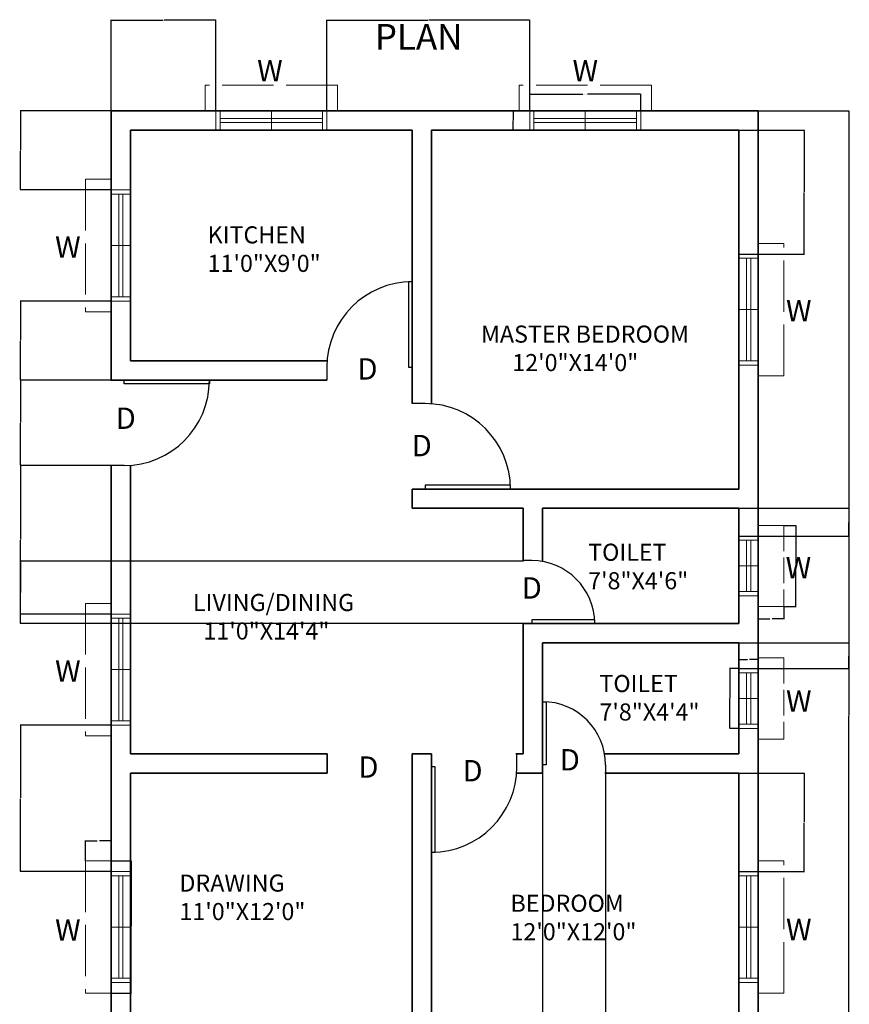
# Model space of a CAD drawing. Units: inches. Extents: x -154 to 668, y -797 to 97.
# Tile 3 of 4: x -115 to 274, y -367 to 94. Entities that reach past the tile are written whole.
import ezdxf

# ---------------------------------------------------------------- set-up
doc = ezdxf.new("R2010")
doc.units = ezdxf.units.IN
doc.header["$MEASUREMENT"] = 0
doc.linetypes.add('ACAD_ISO02W100', pattern=[15, 12, -3])
for name, color, linetype, lineweight in [('A-ANNO-DIMS', 2, 'Continuous', 18), ('A-ANNO-IDEN', 7, 'Continuous', 18), ('A-ANNO-TITL', 1, 'Continuous', 30), ('A-AREA-IDEN', 7, 'Continuous', 18), ('A-DOOR', 7, 'Continuous', 25), ('A-GLAZ', 220, 'Continuous', 18), ('A-GLAZ-OVHD', 220, 'ACAD_ISO02W100', 13), ('A-WALL', 4, 'Continuous', 35)]:
    doc.layers.add(name, color=color, linetype=linetype, lineweight=lineweight)
doc.styles.get("Standard").update_dxf_attribs({"font": 'arial.ttf'})
doc.dimstyles.get("Standard").update_dxf_attribs({"dimtxt": 0.18, "dimasz": 0.18, "dimexe": 0.18, "dimexo": 0.0625, "dimgap": 0.09, "dimtad": 0, "dimtih": 1, "dimtoh": 1, "dimdec": 1, "dimzin": 0, "dimdsep": 46, "dimlunit": 4, "dimtxsty": 'Standard', "dimcen": 0.09, "dimadec": 0, "dimazin": 0, "dimtfac": 1, "dimtdec": 1, "dimtofl": 0, "dimtmove": 0, "dimatfit": 3, "dimfxl": 1, "dimtolj": 1, "dimtzin": 0, "dimarcsym": 0})

# ---------------------------------------------------------------- blocks, each defined once
blk = doc.blocks.new('*U2')
for p, q in [((0, 0), (0, -6)), ((-40, 0), (-40, -6))]:
    blk.add_line(p, q)
blk.add_lwpolyline([(0, 0), (0, 40), (-1.75, 40), (-1.75, 0)], close=True)
blk.add_arc((0, 0), 40, 90, 180)
blk = doc.blocks.new('*U4')
for p, q in [((-750, 0), (-750, -100)), ((0, 0), (0, -100))]:
    blk.add_line(p, q)
blk.add_lwpolyline([(0, 0), (0, 750), (-43.75, 750), (-43.75, 0)], close=True)
blk.add_arc((0, 0), 750, 90, 180)
blk = doc.blocks.new('*U5')
for p, q in [((0, 0), (0, -100)), ((750, 0), (750, -100))]:
    blk.add_line(p, q)
blk.add_lwpolyline([(0, 0), (0, 750), (43.75, 750), (43.75, 0)], close=True)
blk.add_arc((0, 0), 750, 0, 90)
blk = doc.blocks.new('*U6')
for p, q in [((0, 0), (0, 6)), ((40, 0), (40, 6))]:
    blk.add_line(p, q)
blk.add_lwpolyline([(0, 0), (0, -40), (1.75, -40), (1.75, 0)], close=True)
blk.add_arc((0, 0), 40, 270, 360)
blk = doc.blocks.new('*U7')
for p, q in [((0, 0), (0, -6)), ((40, 0), (40, -6))]:
    blk.add_line(p, q)
blk.add_lwpolyline([(0, 0), (0, 40), (1.75, 40), (1.75, 0)], close=True)
blk.add_arc((0, 0), 40, 0, 90)
blk = doc.blocks.new('WINDOW-48IN')
for p, q in [((-26, -4.5), (-26, 4.5)), ((-24, -4.5), (-24, 4.5)), ((-24, 1), (24, 1)), ((0, -4.5), (0, 4.5)), ((24, -4.5), (24, 4.5)), ((26, -4.5), (26, 4.5)), ((-24, -1), (24, -1))]:
    blk.add_line(p, q)
blk = doc.blocks.new('WINDOW-SHADE-48IN')
at = {"ltscale": 2}
for p, q in [((-31, -6), (-31, 6)), ((31, 6), (-31, 6)), ((31, -6), (31, 6)), ((-26, -6), (-31, -6)), ((26, -6), (31, -6))]:
    blk.add_line(p, q, dxfattribs=at)
blk = doc.blocks.new('WINDOW-24IN')
for p, q in [((-4.5, 14), (4.5, 14)), ((-4.5, 12), (4.5, 12)), ((-1, 12), (-1, -12)), ((1, 12), (1, -12)), ((-4.5, 0), (4.5, 0)), ((-4.5, -12), (4.5, -12)), ((-4.5, -14), (4.5, -14))]:
    blk.add_line(p, q)
blk = doc.blocks.new('WINDOW-SHADE-24IN')
at = {"ltscale": 2}
for p, q in [((-6, 14), (-6, 19)), ((-6, 19), (6, 19)), ((-6, -14), (-6, -19)), ((-6, -19), (6, -19))]:
    blk.add_line(p, q, dxfattribs=at)
blk.add_line((6, 19), (6, -19))
blk = doc.blocks.new('*D15')
at = {"layer": 'A-ANNO-DIMS', "color": 0, "lineweight": -2, "transparency": 16777216}
for p, q in [((123.8, 51.32), (123.8, 59.24)), ((123.98, 59.06), (148.69, 59.06)), ((175.62, 59.06), (150.92, 59.06)), ((175.8, 51.32), (175.8, 59.24))]:
    blk.add_line(p, q, dxfattribs=at)
at = {"layer": 'A-ANNO-DIMS', "color": 0, "transparency": 16777216}
for points in [[(123.98, 59.09), (123.98, 59.03), (123.8, 59.06)], [(175.62, 59.09), (175.62, 59.03), (175.8, 59.06)]]:
    blk.add_solid(points, dxfattribs=at)
at = {"layer": 'Defpoints', "color": 0, "transparency": 16777216}
for p in [(123.8, 59.06), (123.8, 51.26), (175.8, 51.26)]:
    blk.add_point(p, dxfattribs=at)
at = {"layer": 'A-ANNO-DIMS', "color": 0, "transparency": 16777216, "insert": (149.8, 59.06), "char_height": 0.18, "attachment_point": 5}
blk.add_mtext('\\A1;WINDOW 52 TYP.', dxfattribs=at)
blk = doc.blocks.new('*D16')
at = {"layer": 'A-ANNO-DIMS', "color": 0, "lineweight": -2, "transparency": 16777216}
for p, q in [((123.74, 51.26), (115.82, 51.26)), ((116, 51.08), (116, 46.94)), ((116, 42.44), (116, 46.58)), ((123.74, 42.26), (115.82, 42.26))]:
    blk.add_line(p, q, dxfattribs=at)
at = {"layer": 'A-ANNO-DIMS', "color": 0, "transparency": 16777216}
for points in [[(115.97, 51.08), (116.03, 51.08), (116, 51.26)], [(115.97, 42.44), (116.03, 42.44), (116, 42.26)]]:
    blk.add_solid(points, dxfattribs=at)
at = {"layer": 'Defpoints', "color": 0, "transparency": 16777216}
for p in [(123.8, 51.26), (116, 42.26), (123.8, 42.26)]:
    blk.add_point(p, dxfattribs=at)
at = {"layer": 'A-ANNO-DIMS', "color": 0, "transparency": 16777216, "insert": (116, 46.76), "char_height": 0.18, "attachment_point": 5}
blk.add_mtext('\\A1;9 TYP.', dxfattribs=at)
blk = doc.blocks.new('*D17')
at = {"layer": 'A-ANNO-DIMS', "color": 0, "lineweight": -2, "transparency": 16777216}
for p, q in [((-72.13, -299.74), (-62.72, -299.74)), ((-62.9, -299.92), (-62.9, -330.56)), ((-62.9, -361.56), (-62.9, -330.92)), ((-72.13, -361.74), (-62.72, -361.74))]:
    blk.add_line(p, q, dxfattribs=at)
at = {"layer": 'A-ANNO-DIMS', "color": 0, "transparency": 16777216}
for points in [[(-62.93, -299.92), (-62.87, -299.92), (-62.9, -299.74)], [(-62.93, -361.56), (-62.87, -361.56), (-62.9, -361.74)]]:
    blk.add_solid(points, dxfattribs=at)
at = {"layer": 'Defpoints', "color": 0, "transparency": 16777216}
for p in [(-72.2, -299.74), (-62.9, -299.74), (-72.2, -361.74)]:
    blk.add_point(p, dxfattribs=at)
at = {"layer": 'A-ANNO-DIMS', "color": 0, "transparency": 16777216, "insert": (-62.9, -330.74), "char_height": 0.18, "attachment_point": 5}
blk.add_mtext('\\A1;SHADE 62 TYP.', dxfattribs=at)
blk = doc.blocks.new('*D18')
at = {"layer": 'A-ANNO-DIMS', "color": 0, "lineweight": -2, "transparency": 16777216}
for p, q in [((-84.2, -299.68), (-84.2, -290.26)), ((-72.2, -299.68), (-72.2, -290.26)), ((-84.02, -290.44), (-78.72, -290.44)), ((-72.38, -290.44), (-77.68, -290.44))]:
    blk.add_line(p, q, dxfattribs=at)
at = {"layer": 'A-ANNO-DIMS', "color": 0, "transparency": 16777216}
for points in [[(-84.02, -290.41), (-84.02, -290.47), (-84.2, -290.44)], [(-72.38, -290.41), (-72.38, -290.47), (-72.2, -290.44)]]:
    blk.add_solid(points, dxfattribs=at)
at = {"layer": 'Defpoints', "color": 0, "transparency": 16777216}
for p in [(-84.2, -290.44), (-84.2, -299.74), (-72.2, -299.74)]:
    blk.add_point(p, dxfattribs=at)
at = {"layer": 'A-ANNO-DIMS', "color": 0, "transparency": 16777216, "insert": (-78.2, -290.44), "char_height": 0.18, "attachment_point": 5}
blk.add_mtext('\\A1;12 TYP.', dxfattribs=at)
blk = doc.blocks.new('*D19')
at = {"layer": 'A-ANNO-DIMS', "color": 0, "lineweight": -2, "transparency": 16777216}
for p, q in [((221.74, -209.74), (217.42, -209.74)), ((217.6, -209.92), (217.6, -223.56)), ((217.6, -237.56), (217.6, -223.92)), ((221.74, -237.74), (217.42, -237.74))]:
    blk.add_line(p, q, dxfattribs=at)
at = {"layer": 'A-ANNO-DIMS', "color": 0, "transparency": 16777216}
for points in [[(217.57, -209.92), (217.63, -209.92), (217.6, -209.74)], [(217.57, -237.56), (217.63, -237.56), (217.6, -237.74)]]:
    blk.add_solid(points, dxfattribs=at)
at = {"layer": 'Defpoints', "color": 0, "transparency": 16777216}
for p in [(217.6, -209.74), (221.8, -209.74), (221.8, -237.74)]:
    blk.add_point(p, dxfattribs=at)
at = {"layer": 'A-ANNO-DIMS', "color": 0, "transparency": 16777216, "insert": (217.6, -223.74), "char_height": 0.18, "attachment_point": 5}
blk.add_mtext('\\A1;WINDOW 28 TYP.', dxfattribs=at)
blk = doc.blocks.new('*D20')
at = {"layer": 'A-ANNO-DIMS', "color": 0, "lineweight": -2, "transparency": 16777216}
for p, q in [((221.8, -209.68), (221.8, -205.36)), ((221.98, -205.54), (225.85, -205.54)), ((230.62, -205.54), (226.76, -205.54)), ((230.8, -209.68), (230.8, -205.36))]:
    blk.add_line(p, q, dxfattribs=at)
at = {"layer": 'A-ANNO-DIMS', "color": 0, "transparency": 16777216}
for points in [[(221.98, -205.51), (221.98, -205.57), (221.8, -205.54)], [(230.62, -205.51), (230.62, -205.57), (230.8, -205.54)]]:
    blk.add_solid(points, dxfattribs=at)
at = {"layer": 'Defpoints', "color": 0, "transparency": 16777216}
for p in [(230.8, -205.54), (221.8, -209.74), (230.8, -209.74)]:
    blk.add_point(p, dxfattribs=at)
at = {"layer": 'A-ANNO-DIMS', "color": 0, "transparency": 16777216, "insert": (226.3, -205.54), "char_height": 0.18, "attachment_point": 5}
blk.add_mtext('\\A1;9 TYP.', dxfattribs=at)
blk = doc.blocks.new('*D21')
at = {"layer": 'A-ANNO-DIMS', "color": 0, "lineweight": -2, "transparency": 16777216}
for p, q in [((242.87, -142.74), (248.68, -142.74)), ((248.5, -142.92), (248.5, -161.56)), ((248.5, -180.56), (248.5, -161.92)), ((242.87, -180.74), (248.68, -180.74))]:
    blk.add_line(p, q, dxfattribs=at)
at = {"layer": 'A-ANNO-DIMS', "color": 0, "transparency": 16777216}
for points in [[(248.47, -142.92), (248.53, -142.92), (248.5, -142.74)], [(248.47, -180.56), (248.53, -180.56), (248.5, -180.74)]]:
    blk.add_solid(points, dxfattribs=at)
at = {"layer": 'Defpoints', "color": 0, "transparency": 16777216}
for p in [(242.8, -142.74), (248.5, -142.74), (242.8, -180.74)]:
    blk.add_point(p, dxfattribs=at)
at = {"layer": 'A-ANNO-DIMS', "color": 0, "transparency": 16777216, "insert": (248.5, -161.74), "char_height": 0.18, "attachment_point": 5}
blk.add_mtext('\\A1;SHADE 38 TYP.', dxfattribs=at)
blk = doc.blocks.new('*D22')
at = {"layer": 'A-ANNO-DIMS', "color": 0, "lineweight": -2, "transparency": 16777216}
for p, q in [((230.8, -180.8), (230.8, -186.62)), ((242.8, -180.8), (242.8, -186.62)), ((230.98, -186.44), (236.28, -186.44)), ((242.62, -186.44), (237.32, -186.44))]:
    blk.add_line(p, q, dxfattribs=at)
at = {"layer": 'A-ANNO-DIMS', "color": 0, "transparency": 16777216}
for points in [[(230.98, -186.41), (230.98, -186.47), (230.8, -186.44)], [(242.62, -186.41), (242.62, -186.47), (242.8, -186.44)]]:
    blk.add_solid(points, dxfattribs=at)
at = {"layer": 'Defpoints', "color": 0, "transparency": 16777216}
for p in [(230.8, -180.74), (242.8, -180.74), (242.8, -186.44)]:
    blk.add_point(p, dxfattribs=at)
at = {"layer": 'A-ANNO-DIMS', "color": 0, "transparency": 16777216, "insert": (236.8, -186.44), "char_height": 0.18, "attachment_point": 5}
blk.add_mtext('\\A1;12 TYP.', dxfattribs=at)
blk = doc.blocks.new('*D28')
at = {"layer": 'A-ANNO-DIMS', "color": 0, "lineweight": -2, "transparency": 16777216}
for p, q in [((230.87, 51.26), (273.48, 51.26)), ((273.3, 51.08), (273.3, -231.56)), ((273.3, -514.56), (273.3, -231.92)), ((230.87, -514.74), (273.48, -514.74))]:
    blk.add_line(p, q, dxfattribs=at)
at = {"layer": 'A-ANNO-DIMS', "color": 0, "transparency": 16777216}
for points in [[(273.27, 51.08), (273.33, 51.08), (273.3, 51.26)], [(273.27, -514.56), (273.33, -514.56), (273.3, -514.74)]]:
    blk.add_solid(points, dxfattribs=at)
at = {"layer": 'Defpoints', "color": 0, "transparency": 16777216}
for p in [(230.8, 51.26), (273.3, 51.26), (230.8, -514.74)]:
    blk.add_point(p, dxfattribs=at)
at = {"layer": 'A-ANNO-DIMS', "color": 0, "transparency": 16777216, "insert": (273.3, -231.74), "char_height": 0.18, "attachment_point": 5}
blk.add_mtext('\\A1;566', dxfattribs=at)
blk = doc.blocks.new('*D30')
at = {"layer": 'A-ANNO-DIMS', "color": 0, "lineweight": -2, "transparency": 16777216}
for p, q in [((-72.2, 51.32), (-72.2, 93.94)), ((-72.02, 93.76), (-47.92, 93.76)), ((-23.38, 93.76), (-47.47, 93.76)), ((-23.2, 51.32), (-23.2, 93.94))]:
    blk.add_line(p, q, dxfattribs=at)
at = {"layer": 'A-ANNO-DIMS', "color": 0, "transparency": 16777216}
for points in [[(-72.02, 93.79), (-72.02, 93.73), (-72.2, 93.76)], [(-23.38, 93.79), (-23.38, 93.73), (-23.2, 93.76)]]:
    blk.add_solid(points, dxfattribs=at)
at = {"layer": 'Defpoints', "color": 0, "transparency": 16777216}
for p in [(-72.2, 93.76), (-72.2, 51.26), (-23.2, 51.26)]:
    blk.add_point(p, dxfattribs=at)
at = {"layer": 'A-ANNO-DIMS', "color": 0, "transparency": 16777216, "insert": (-47.7, 93.76), "char_height": 0.18, "attachment_point": 5}
blk.add_mtext('\\A1;49', dxfattribs=at)
blk = doc.blocks.new('*D31')
at = {"layer": 'A-ANNO-DIMS', "color": 0, "lineweight": -2, "transparency": 16777216}
for p, q in [((28.8, 51.32), (28.8, 93.94)), ((28.98, 93.76), (76.08, 93.76)), ((123.62, 93.76), (76.52, 93.76)), ((123.8, 51.32), (123.8, 93.94))]:
    blk.add_line(p, q, dxfattribs=at)
at = {"layer": 'A-ANNO-DIMS', "color": 0, "transparency": 16777216}
for points in [[(28.98, 93.79), (28.98, 93.73), (28.8, 93.76)], [(123.62, 93.79), (123.62, 93.73), (123.8, 93.76)]]:
    blk.add_solid(points, dxfattribs=at)
at = {"layer": 'Defpoints', "color": 0, "transparency": 16777216}
for p in [(123.8, 93.76), (28.8, 51.26), (123.8, 51.26)]:
    blk.add_point(p, dxfattribs=at)
at = {"layer": 'A-ANNO-DIMS', "color": 0, "transparency": 16777216, "insert": (76.3, 93.76), "char_height": 0.18, "attachment_point": 5}
blk.add_mtext('\\A1;95', dxfattribs=at)
blk = doc.blocks.new('*D32')
at = {"layer": 'A-ANNO-DIMS', "color": 0, "lineweight": -2, "transparency": 16777216}
for p, q in [((-72.26, 51.26), (-114.88, 51.26)), ((-114.7, 51.08), (-114.7, 32.94)), ((-114.7, 14.44), (-114.7, 32.58)), ((-72.26, 14.26), (-114.88, 14.26))]:
    blk.add_line(p, q, dxfattribs=at)
at = {"layer": 'A-ANNO-DIMS', "color": 0, "transparency": 16777216}
for points in [[(-114.73, 51.08), (-114.67, 51.08), (-114.7, 51.26)], [(-114.73, 14.44), (-114.67, 14.44), (-114.7, 14.26)]]:
    blk.add_solid(points, dxfattribs=at)
at = {"layer": 'Defpoints', "color": 0, "transparency": 16777216}
for p in [(-72.2, 51.26), (-114.7, 14.26), (-72.2, 14.26)]:
    blk.add_point(p, dxfattribs=at)
at = {"layer": 'A-ANNO-DIMS', "color": 0, "transparency": 16777216, "insert": (-114.7, 32.76), "char_height": 0.18, "attachment_point": 5}
blk.add_mtext('\\A1;37', dxfattribs=at)
blk = doc.blocks.new('*D33')
at = {"layer": 'A-ANNO-DIMS', "color": 0, "lineweight": -2, "transparency": 16777216}
for p, q in [((-72.26, -37.74), (-114.88, -37.74)), ((-114.7, -37.92), (-114.7, -56.06)), ((-114.7, -74.56), (-114.7, -56.42)), ((-72.26, -74.74), (-114.88, -74.74))]:
    blk.add_line(p, q, dxfattribs=at)
at = {"layer": 'A-ANNO-DIMS', "color": 0, "transparency": 16777216}
for points in [[(-114.73, -37.92), (-114.67, -37.92), (-114.7, -37.74)], [(-114.73, -74.56), (-114.67, -74.56), (-114.7, -74.74)]]:
    blk.add_solid(points, dxfattribs=at)
at = {"layer": 'Defpoints', "color": 0, "transparency": 16777216}
for p in [(-72.2, -37.74), (-114.7, -74.74), (-72.2, -74.74)]:
    blk.add_point(p, dxfattribs=at)
at = {"layer": 'A-ANNO-DIMS', "color": 0, "transparency": 16777216, "insert": (-114.7, -56.24), "char_height": 0.18, "attachment_point": 5}
blk.add_mtext('\\A1;37', dxfattribs=at)
blk = doc.blocks.new('*D34')
at = {"layer": 'A-ANNO-DIMS', "color": 0, "lineweight": -2, "transparency": 16777216}
for p, q in [((-72.26, -74.74), (-114.88, -74.74)), ((-114.7, -74.92), (-114.7, -94.56)), ((-114.7, -114.56), (-114.7, -94.92)), ((-72.26, -114.74), (-114.88, -114.74))]:
    blk.add_line(p, q, dxfattribs=at)
at = {"layer": 'A-ANNO-DIMS', "color": 0, "transparency": 16777216}
for points in [[(-114.73, -74.92), (-114.67, -74.92), (-114.7, -74.74)], [(-114.73, -114.56), (-114.67, -114.56), (-114.7, -114.74)]]:
    blk.add_solid(points, dxfattribs=at)
at = {"layer": 'Defpoints', "color": 0, "transparency": 16777216}
for p in [(-72.2, -74.74), (-114.7, -114.74), (-72.2, -114.74)]:
    blk.add_point(p, dxfattribs=at)
at = {"layer": 'A-ANNO-DIMS', "color": 0, "transparency": 16777216, "insert": (-114.7, -94.74), "char_height": 0.18, "attachment_point": 5}
blk.add_mtext('\\A1;40', dxfattribs=at)
blk = doc.blocks.new('*D35')
at = {"layer": 'A-ANNO-DIMS', "color": 0, "lineweight": -2, "transparency": 16777216}
for p, q in [((-72.26, -114.74), (-114.88, -114.74)), ((-114.7, -114.92), (-114.7, -149.31)), ((-114.7, -184.06), (-114.7, -149.67)), ((-72.26, -184.24), (-114.88, -184.24))]:
    blk.add_line(p, q, dxfattribs=at)
at = {"layer": 'A-ANNO-DIMS', "color": 0, "transparency": 16777216}
for points in [[(-114.73, -114.92), (-114.67, -114.92), (-114.7, -114.74)], [(-114.73, -184.06), (-114.67, -184.06), (-114.7, -184.24)]]:
    blk.add_solid(points, dxfattribs=at)
at = {"layer": 'Defpoints', "color": 0, "transparency": 16777216}
for p in [(-72.2, -114.74), (-114.7, -184.24), (-72.2, -184.24)]:
    blk.add_point(p, dxfattribs=at)
at = {"layer": 'A-ANNO-DIMS', "color": 0, "transparency": 16777216, "insert": (-114.7, -149.49), "char_height": 0.18, "attachment_point": 5}
blk.add_mtext('\\A1;69.5', dxfattribs=at)
blk = doc.blocks.new('*D36')
at = {"layer": 'A-ANNO-DIMS', "color": 0, "lineweight": -2, "transparency": 16777216}
for p, q in [((-72.26, -236.24), (-114.88, -236.24)), ((-114.7, -236.42), (-114.7, -270.31)), ((-114.7, -304.56), (-114.7, -270.67)), ((-72.26, -304.74), (-114.88, -304.74))]:
    blk.add_line(p, q, dxfattribs=at)
at = {"layer": 'A-ANNO-DIMS', "color": 0, "transparency": 16777216}
for points in [[(-114.73, -236.42), (-114.67, -236.42), (-114.7, -236.24)], [(-114.73, -304.56), (-114.67, -304.56), (-114.7, -304.74)]]:
    blk.add_solid(points, dxfattribs=at)
at = {"layer": 'Defpoints', "color": 0, "transparency": 16777216}
for p in [(-72.2, -236.24), (-114.7, -304.74), (-72.2, -304.74)]:
    blk.add_point(p, dxfattribs=at)
at = {"layer": 'A-ANNO-DIMS', "color": 0, "transparency": 16777216, "insert": (-114.7, -270.49), "char_height": 0.18, "attachment_point": 5}
blk.add_mtext('\\A1;68.5', dxfattribs=at)
blk = doc.blocks.new('*D37')
at = {"layer": 'A-ANNO-DIMS', "color": 0, "lineweight": -2, "transparency": 16777216}
for p, q in [((120.74, -159.48), (-114.88, -159.48)), ((-114.7, -159.66), (-114.7, -173.93)), ((-114.7, -188.56), (-114.7, -174.29)), ((120.74, -188.74), (-114.88, -188.74))]:
    blk.add_line(p, q, dxfattribs=at)
at = {"layer": 'A-ANNO-DIMS', "color": 0, "transparency": 16777216}
for points in [[(-114.73, -159.66), (-114.67, -159.66), (-114.7, -159.48)], [(-114.73, -188.56), (-114.67, -188.56), (-114.7, -188.74)]]:
    blk.add_solid(points, dxfattribs=at)
at = {"layer": 'Defpoints', "color": 0, "transparency": 16777216}
for p in [(120.8, -159.48), (-114.7, -188.74), (120.8, -188.74)]:
    blk.add_point(p, dxfattribs=at)
at = {"layer": 'A-ANNO-DIMS', "color": 0, "transparency": 16777216, "insert": (-114.7, -174.11), "char_height": 0.18, "attachment_point": 5}
blk.add_mtext('\\A1;29.264', dxfattribs=at)
blk = doc.blocks.new('*D38')
at = {"layer": 'A-ANNO-DIMS', "color": 0, "lineweight": -2, "transparency": 16777216}
for p, q in [((129.8, -258.8), (129.8, -545.42)), ((159.33, -258.8), (159.33, -545.42)), ((129.98, -545.24), (144.17, -545.24)), ((159.15, -545.24), (144.96, -545.24))]:
    blk.add_line(p, q, dxfattribs=at)
at = {"layer": 'A-ANNO-DIMS', "color": 0, "transparency": 16777216}
for points in [[(129.98, -545.21), (129.98, -545.27), (129.8, -545.24)], [(159.15, -545.21), (159.15, -545.27), (159.33, -545.24)]]:
    blk.add_solid(points, dxfattribs=at)
at = {"layer": 'Defpoints', "color": 0, "transparency": 16777216}
for p in [(129.8, -258.74), (159.33, -258.74), (159.33, -545.24)]:
    blk.add_point(p, dxfattribs=at)
at = {"layer": 'A-ANNO-DIMS', "color": 0, "transparency": 16777216, "insert": (144.57, -545.24), "char_height": 0.18, "attachment_point": 5}
blk.add_mtext('\\A1;29.53', dxfattribs=at)
blk = doc.blocks.new('*D39')
at = {"layer": 'A-ANNO-DIMS', "color": 0, "lineweight": -2, "transparency": 16777216}
for p, q in [((221.87, 42.26), (252.48, 42.26)), ((252.3, 42.08), (252.3, 13.44)), ((252.3, -15.56), (252.3, 13.08)), ((221.87, -15.74), (252.48, -15.74))]:
    blk.add_line(p, q, dxfattribs=at)
at = {"layer": 'A-ANNO-DIMS', "color": 0, "transparency": 16777216}
for points in [[(252.27, 42.08), (252.33, 42.08), (252.3, 42.26)], [(252.27, -15.56), (252.33, -15.56), (252.3, -15.74)]]:
    blk.add_solid(points, dxfattribs=at)
at = {"layer": 'Defpoints', "color": 0, "transparency": 16777216}
for p in [(221.8, 42.26), (221.8, -15.74), (252.3, -15.74)]:
    blk.add_point(p, dxfattribs=at)
at = {"layer": 'A-ANNO-DIMS', "color": 0, "transparency": 16777216, "insert": (252.3, 13.26), "char_height": 0.18, "attachment_point": 5}
blk.add_mtext('\\A1;58', dxfattribs=at)
blk = doc.blocks.new('*D40')
at = {"layer": 'A-ANNO-DIMS', "color": 0, "lineweight": -2, "transparency": 16777216}
for p, q in [((221.87, -134.74), (273.48, -134.74)), ((273.3, -134.92), (273.3, -141.06)), ((273.3, -147.56), (273.3, -141.42)), ((221.87, -147.74), (273.48, -147.74))]:
    blk.add_line(p, q, dxfattribs=at)
at = {"layer": 'A-ANNO-DIMS', "color": 0, "transparency": 16777216}
for points in [[(273.27, -134.92), (273.33, -134.92), (273.3, -134.74)], [(273.27, -147.56), (273.33, -147.56), (273.3, -147.74)]]:
    blk.add_solid(points, dxfattribs=at)
at = {"layer": 'Defpoints', "color": 0, "transparency": 16777216}
for p in [(221.8, -134.74), (273.3, -134.74), (221.8, -147.74)]:
    blk.add_point(p, dxfattribs=at)
at = {"layer": 'A-ANNO-DIMS', "color": 0, "transparency": 16777216, "insert": (273.3, -141.24), "char_height": 0.18, "attachment_point": 5}
blk.add_mtext('\\A1;13', dxfattribs=at)
blk = doc.blocks.new('*D41')
at = {"layer": 'A-ANNO-DIMS', "color": 0, "lineweight": -2, "transparency": 16777216}
for p, q in [((221.87, -197.74), (273.48, -197.74)), ((273.3, -197.92), (273.3, -203.56)), ((273.3, -209.56), (273.3, -203.92)), ((221.87, -209.74), (273.48, -209.74))]:
    blk.add_line(p, q, dxfattribs=at)
at = {"layer": 'A-ANNO-DIMS', "color": 0, "transparency": 16777216}
for points in [[(273.27, -197.92), (273.33, -197.92), (273.3, -197.74)], [(273.27, -209.56), (273.33, -209.56), (273.3, -209.74)]]:
    blk.add_solid(points, dxfattribs=at)
at = {"layer": 'Defpoints', "color": 0, "transparency": 16777216}
for p in [(221.8, -197.74), (273.3, -197.74), (221.8, -209.74)]:
    blk.add_point(p, dxfattribs=at)
at = {"layer": 'A-ANNO-DIMS', "color": 0, "transparency": 16777216, "insert": (273.3, -203.74), "char_height": 0.18, "attachment_point": 5}
blk.add_mtext('\\A1;12', dxfattribs=at)
blk = doc.blocks.new('*D42')
at = {"layer": 'A-ANNO-DIMS', "color": 0, "lineweight": -2, "transparency": 16777216}
for p, q in [((221.87, -258.74), (252.48, -258.74)), ((252.3, -258.92), (252.3, -281.56)), ((252.3, -304.56), (252.3, -281.92)), ((221.87, -304.74), (252.48, -304.74))]:
    blk.add_line(p, q, dxfattribs=at)
at = {"layer": 'A-ANNO-DIMS', "color": 0, "transparency": 16777216}
for points in [[(252.27, -258.92), (252.33, -258.92), (252.3, -258.74)], [(252.27, -304.56), (252.33, -304.56), (252.3, -304.74)]]:
    blk.add_solid(points, dxfattribs=at)
at = {"layer": 'Defpoints', "color": 0, "transparency": 16777216}
for p in [(221.8, -258.74), (221.8, -304.74), (252.3, -304.74)]:
    blk.add_point(p, dxfattribs=at)
at = {"layer": 'A-ANNO-DIMS', "color": 0, "transparency": 16777216, "insert": (252.3, -281.74), "char_height": 0.18, "attachment_point": 5}
blk.add_mtext('\\A1;46', dxfattribs=at)

msp = doc.modelspace()

# ---------------------------------------------------------------- linework, layer by layer
at = {"layer": 'A-WALL'}
for p, q in [((-72.1956, 51.2584), (77.8044, 51.2584)), ((-72.1956, -74.7416), (-72.1956, 51.2584)), ((77.8044, 51.2584), (230.8044, 51.2584)), ((230.8044, 51.2584), (230.8044, -134.7416)), ((-63.1956, 42.2584), (68.8044, 42.2584)), ((-63.1956, -65.7416), (-63.1956, 42.2584)), ((68.8044, 42.2584), (68.8044, -65.7416)), ((68.8044, -85.7416), (68.8044, 42.2584)), ((77.8044, 42.2584), (221.8044, 42.2584)), ((77.8044, -85.8542), (77.8044, 42.2584)), ((221.8044, 42.2584), (221.8044, -125.7416)), ((28.917, -65.7416), (-63.1956, -65.7416)), ((68.8044, -65.7416), (68.8044, -74.7416)), ((28.8044, -74.7416), (-72.1956, -74.7416)), ((-72.1956, -114.7416), (-72.1956, -258.7416)), ((-63.1956, -114.6289), (-63.1956, -249.7416)), ((77.8044, -125.7416), (68.8044, -125.7416)), ((68.8044, -125.7416), (68.8044, -134.7416)), ((221.8044, -125.7416), (77.8044, -125.7416)), ((120.8044, -134.7416), (68.8044, -134.7416)), ((120.8044, -159.4777), (120.8044, -134.7416)), ((221.8044, -134.7416), (129.8044, -134.7416)), ((129.8044, -159.6513), (129.8044, -134.7416)), ((221.8044, -134.7416), (221.8044, -188.7416)), ((230.8044, -134.7416), (230.8044, -197.7416)), ((221.8044, -188.7416), (120.8044, -188.7416)), ((120.8044, -249.7416), (120.8044, -188.7416)), ((221.8044, -197.7416), (129.8044, -197.7416)), ((129.8044, -258.7416), (129.8044, -197.7416)), ((221.8044, -197.7416), (221.8044, -249.7416)), ((230.8044, -197.7416), (230.8044, -258.7416)), ((-63.1956, -249.7416), (28.917, -249.7416)), ((28.917, -258.7416), (28.917, -249.7416)), ((68.8044, -411.7416), (68.8044, -249.7416)), ((68.8044, -249.7416), (77.8044, -249.7416)), ((77.8044, -402.7416), (77.8044, -249.7416)), ((117.3518, -249.7416), (120.8044, -249.7416)), ((221.8044, -249.7416), (158.8946, -249.7416)), ((158.8946, -249.7416), (221.8044, -249.7416)), ((-72.1956, -258.7416), (-72.1956, -411.7416)), ((-63.1956, -258.7416), (28.917, -258.7416)), ((-63.1956, -258.7416), (-63.1956, -402.7416)), ((117.6917, -258.7416), (129.8044, -258.7416)), ((117.6917, -258.7416), (129.8044, -258.7416)), ((159.0683, -258.7416), (221.8044, -258.7416)), ((159.0683, -258.7416), (221.8044, -258.7416)), ((221.8044, -258.7416), (221.8044, -402.7416)), ((230.8044, -258.7416), (230.8044, -514.7416))]:
    msp.add_line(p, q, dxfattribs=at)

# ---------------------------------------------------------------- block references
at = {"layer": 'A-DOOR'}
for name, p in [('*U2', (68.8044, -68.7416)), ('*U6', (77.8044, -255.7416))]:
    msp.add_blockref(name, p, dxfattribs=at)
at = {"layer": 'A-DOOR', "rotation": 270}
for name, p in [('*U7', (-66.1956, -74.7416)), ('*U2', (74.8044, -125.7416))]:
    msp.add_blockref(name, p, dxfattribs=at)
at = {"layer": 'A-DOOR', "xscale": 0.0393700787401575, "yscale": 0.0393700787401575, "zscale": 0.0393700787401575, "rotation": 270}
msp.add_blockref('*U4', (124.7414, -188.7416), dxfattribs=at)
at = {"layer": 'A-DOOR', "xscale": 0.0393700787401575, "yscale": 0.0393700787401575, "zscale": 0.0393700787401575}
msp.add_blockref('*U5', (129.8044, -254.8046), dxfattribs=at)
at = {"layer": 'A-GLAZ'}
for name, p in [('WINDOW-48IN', (2.804, 46.758)), ('WINDOW-24IN', (226.304, -161.742)), ('WINDOW-24IN', (226.304, -223.742))]:
    msp.add_blockref(name, p, dxfattribs=at)
for p, rotation in [((149.8048, 46.7588), 180), ((-67.696, -11.7412), 270), ((226.304, -41.7412), 269.9999999999999), ((-67.696, -210.2412), 270), ((-67.696, -330.7412), 270), ((226.304, -330.7412), 269.9999999999999)]:
    msp.add_blockref('WINDOW-48IN', p, dxfattribs=dict(at, rotation=rotation))
at = {"layer": 'A-GLAZ-OVHD'}
for name, p in [('WINDOW-SHADE-48IN', (2.804, 57.258)), ('WINDOW-SHADE-48IN', (149.804, 57.258)), ('WINDOW-SHADE-24IN', (236.804, -161.742)), ('WINDOW-SHADE-24IN', (236.804, -223.742))]:
    msp.add_blockref(name, p, dxfattribs=at)
for p, rotation in [((-78.1952, -11.742), 90.00000000000003), ((236.804, -41.7412), 269.9999999999999), ((-78.1952, -210.242), 90.00000000000003), ((-78.1952, -330.742), 89.99999999999996), ((236.804, -330.7412), 270)]:
    msp.add_blockref('WINDOW-SHADE-48IN', p, dxfattribs=dict(at, rotation=rotation))

# ---------------------------------------------------------------- texts
at = {"layer": 'A-ANNO-IDEN'}
for s, p in [('W', (-3.8477, 65.0991)), ('W', (143.8583, 65.0991)), ('W', (-98.4848, -17.5194)), ('W', (243.86, -47.2239)), ('D', (43.1493, -74.5111)), ('D', (-70.0862, -97.5957)), ('D', (68.5487, -110.4044)), ('W', (243.6708, -167.5442)), ('D', (120.1076, -177.0321)), ('W', (-98.4848, -215.9575)), ('W', (243.86, -229.9583)), ('D', (137.9232, -257.4576)), ('D', (43.5993, -260.8708)), ('D', (92.3647, -262.5655)), ('W', (-98.4848, -337.1226)), ('W', (243.86, -336.8856))]:
    msp.add_text(s, height=10, dxfattribs=at).set_placement(p)
at = {"layer": 'A-ANNO-TITL'}
msp.add_text('PLAN', height=12, dxfattribs=at).set_placement((51.278, 79.9286))
at = {"layer": 'A-AREA-IDEN', "char_height": 8, "attachment_point": 1}
for s, width, insert in [('KITCHEN\\P11\'0"X9\'0"', 87.70688, (-27.0416, -2.7674)), ('MASTER BEDROOM\\P      12\'0"X14\'0"', 149.590108, (100.9798, -49.2125)), ('TOILET\\P7\'8"X4\'6"', 87.70688, (151.172, -151.3151)), ('LIVING/DINING\\P  11\'0"X14\'4"', 87.70688, (-33.8999, -174.8427)), ('TOILET\\P7\'8"X4\'4"', 87.70688, (156.4569, -212.7466)), ('DRAWING\\P11\'0"X12\'0"', 87.70688, (-40.2507, -306.1648)), ('BEDROOM\\P12\'0"X12\'0"', 87.70688, (114.7981, -315.5959))]:
    msp.add_mtext_dynamic_manual_height_columns(s, width=width, gutter_width=1, heights=[0], dxfattribs=dict(at, insert=insert))

# ---------------------------------------------------------------- dimensions: what is measured, and where the dimension line sits
at = {"layer": 'A-ANNO-DIMS'}
for base, p1, p2, override, picture, middle in [((-72.1956, 93.7584), (-23.1956, 51.2584), (-72.1956, 51.2584), {"dimdec": 0, "dimlfac": 1, "dimrnd": 0, "dimzin": 0, "dimdsep": 46, "dimlunit": 2}, '*D30', (-47.6956, 93.7584)), ((123.8044, 93.7584), (28.8044, 51.2584), (123.8044, 51.2584), {"dimdec": 0, "dimlfac": 1, "dimrnd": 0, "dimzin": 0, "dimdsep": 46, "dimlunit": 2}, '*D31', (76.3044, 93.7584)), ((159.3319, -545.2416), (129.8044, -258.7416), (159.3319, -258.7416), {"dimdec": 2, "dimlfac": 1, "dimrnd": 0, "dimzin": 0, "dimdsep": 46, "dimlunit": 2}, '*D38', (144.5682, -545.2416))]:
    dim = msp.add_linear_dim(base=base, p1=p1, p2=p2, dimstyle='Standard', override=override, dxfattribs=at)
    dim.commit()
    dim.dimension.update_dxf_attribs({"geometry": picture, "text_midpoint": middle})
for base, p1, p2, angle, text, picture, middle in [((123.8044, 59.0584), (175.8044, 51.2584), (123.8044, 51.2584), 180, 'WINDOW <> TYP.', '*D15', (149.8044, 59.0584)), ((116.0044, 42.2584), (123.8044, 51.2584), (123.8044, 42.2584), 270, '<> TYP.', '*D16', (116.0044, 46.7584)), ((248.5044, -142.7416), (242.8044, -180.7416), (242.8044, -142.7416), 90, 'SHADE <> TYP.', '*D21', (248.5044, -161.7416)), ((217.6044, -209.7416), (221.8044, -237.7416), (221.8044, -209.7416), 90, 'WINDOW <> TYP.', '*D19', (217.6044, -223.7416)), ((-84.1956, -290.4416), (-72.1956, -299.7416), (-84.1956, -299.7416), 180, '<> TYP.', '*D18', (-78.1956, -290.4416)), ((-62.8956, -299.7416), (-72.1956, -361.7416), (-72.1956, -299.7416), 90, 'SHADE <> TYP.', '*D17', (-62.8956, -330.7416))]:
    dim = msp.add_linear_dim(base=base, p1=p1, p2=p2, angle=angle, text=text, dimstyle='Standard', override={"dimdec": 0, "dimlfac": 1, "dimrnd": 0, "dimzin": 0, "dimdsep": 46, "dimlunit": 2}, dxfattribs=at)
    dim.commit()
    dim.dimension.update_dxf_attribs({"geometry": picture, "text_midpoint": middle})
for base, p1, p2, angle, override, picture, middle in [((-114.6956, 14.2584), (-72.1956, 51.2584), (-72.1956, 14.2584), 90, {"dimdec": 0, "dimlfac": 1, "dimrnd": 0, "dimzin": 0, "dimdsep": 46, "dimlunit": 2}, '*D32', (-114.6956, 32.7584)), ((273.3044, 51.2584), (230.8044, -514.7416), (230.8044, 51.2584), 90, {"dimdec": 0, "dimlfac": 1, "dimrnd": 0, "dimzin": 0, "dimdsep": 46, "dimlunit": 2}, '*D28', (273.3044, -231.7416)), ((252.3044, -15.7416), (221.8044, 42.2584), (221.8044, -15.7416), 270, {"dimdec": 0, "dimlfac": 1, "dimrnd": 0, "dimzin": 0, "dimdsep": 46, "dimlunit": 2}, '*D39', (252.3044, 13.2584)), ((-114.6956, -74.7416), (-72.1956, -37.7416), (-72.1956, -74.7416), 90, {"dimdec": 0, "dimlfac": 1, "dimrnd": 0, "dimzin": 0, "dimdsep": 46, "dimlunit": 2}, '*D33', (-114.6956, -56.2416)), ((-114.6956, -114.7416), (-72.1956, -74.7416), (-72.1956, -114.7416), 90, {"dimdec": 0, "dimlfac": 1, "dimrnd": 0, "dimzin": 0, "dimdsep": 46, "dimlunit": 2}, '*D34', (-114.6956, -94.7416)), ((-114.6956, -184.2416), (-72.1956, -114.7416), (-72.1956, -184.2416), 90, {"dimdec": 1, "dimlfac": 1, "dimrnd": 0, "dimzin": 0, "dimdsep": 46, "dimlunit": 2}, '*D35', (-114.6956, -149.4916)), ((273.3044, -134.7416), (221.8044, -147.7416), (221.8044, -134.7416), 90, {"dimdec": 0, "dimlfac": 1, "dimrnd": 0, "dimzin": 0, "dimdsep": 46, "dimlunit": 2}, '*D40', (273.3044, -141.2416)), ((-114.6956, -188.7416), (120.8044, -159.4777), (120.8044, -188.7416), 90, {"dimdec": 3, "dimlfac": 1, "dimrnd": 0, "dimzin": 0, "dimdsep": 46, "dimlunit": 2}, '*D37', (-114.6956, -174.1096)), ((273.3044, -197.7416), (221.8044, -209.7416), (221.8044, -197.7416), 90, {"dimdec": 0, "dimlfac": 1, "dimrnd": 0, "dimzin": 0, "dimdsep": 46, "dimlunit": 2}, '*D41', (273.3044, -203.7416)), ((-114.6956, -304.7416), (-72.1956, -236.2416), (-72.1956, -304.7416), 90, {"dimdec": 1, "dimlfac": 1, "dimrnd": 0, "dimzin": 0, "dimdsep": 46, "dimlunit": 2}, '*D36', (-114.6956, -270.4916)), ((252.3044, -304.7416), (221.8044, -258.7416), (221.8044, -304.7416), 270, {"dimdec": 0, "dimlfac": 1, "dimrnd": 0, "dimzin": 0, "dimdsep": 46, "dimlunit": 2}, '*D42', (252.3044, -281.7416))]:
    dim = msp.add_linear_dim(base=base, p1=p1, p2=p2, angle=angle, dimstyle='Standard', override=override, dxfattribs=at)
    dim.commit()
    dim.dimension.update_dxf_attribs({"geometry": picture, "text_midpoint": middle})
for base, p1, p2, picture, middle in [((242.8044, -186.4416), (230.8044, -180.7416), (242.8044, -180.7416), '*D22', (236.8044, -186.4416)), ((230.8044, -205.5416), (221.8044, -209.7416), (230.8044, -209.7416), '*D20', (226.3044, -205.5416))]:
    dim = msp.add_linear_dim(base=base, p1=p1, p2=p2, text='<> TYP.', dimstyle='Standard', override={"dimdec": 0, "dimlfac": 1, "dimrnd": 0, "dimzin": 0, "dimdsep": 46, "dimlunit": 2}, dxfattribs=at)
    dim.commit()
    dim.dimension.update_dxf_attribs({"geometry": picture, "text_midpoint": middle})

doc.saveas('drawing.dxf')
